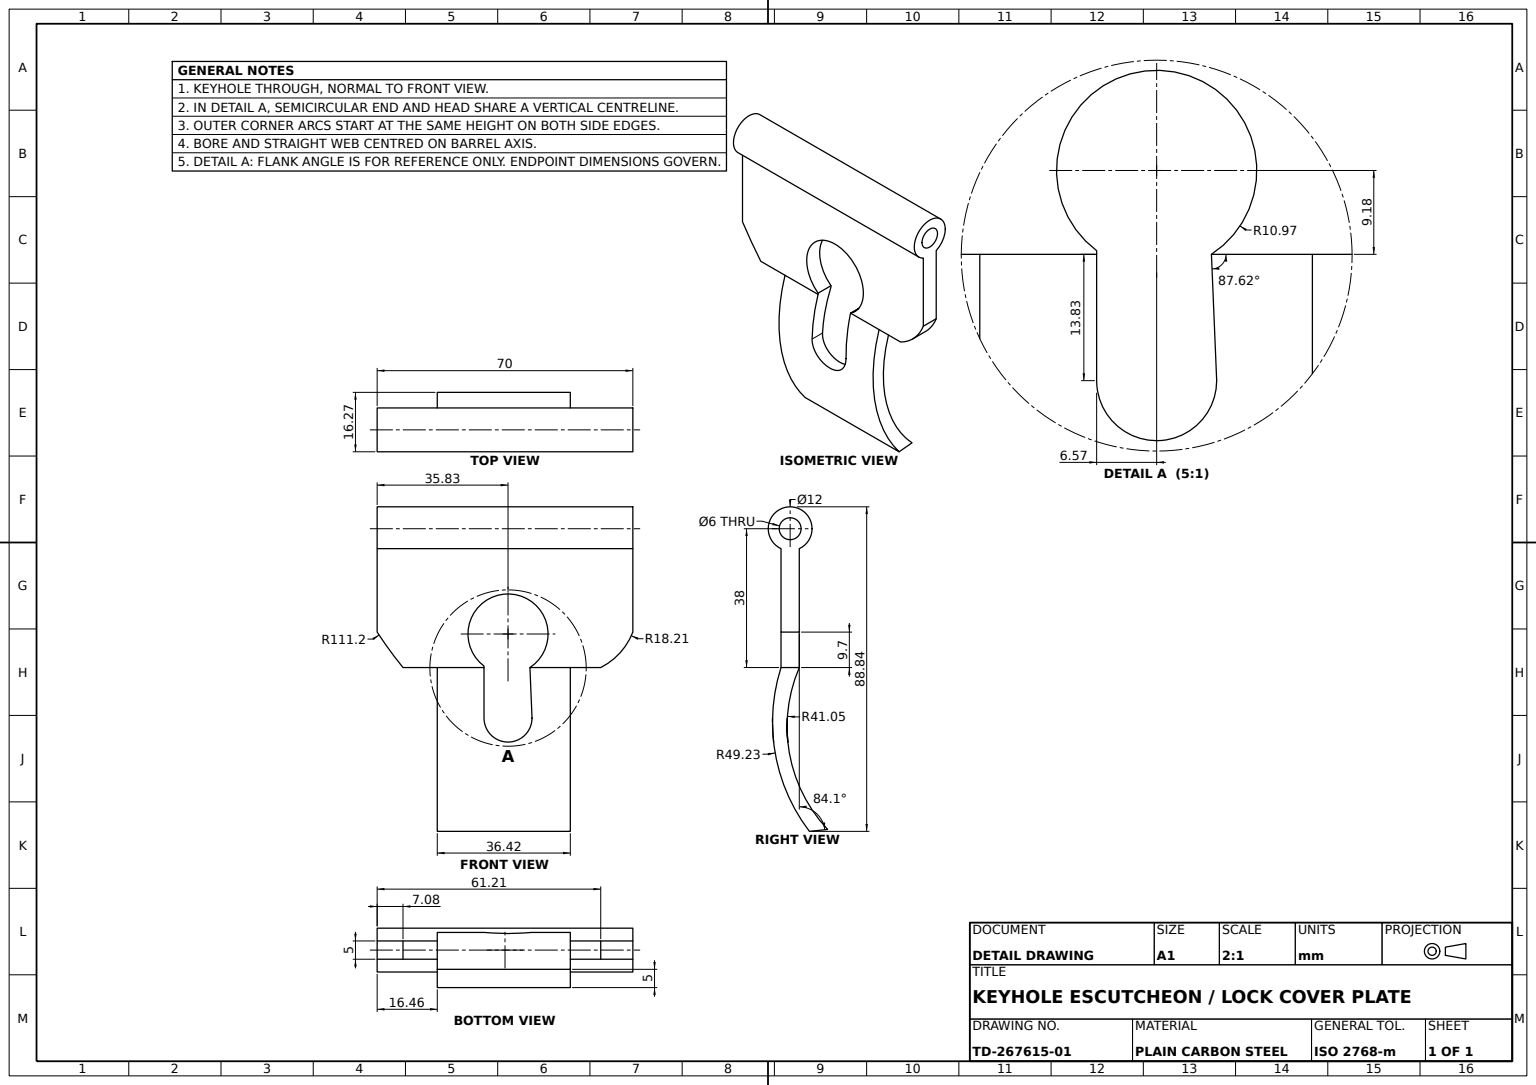
from build123d import *

# Parameters (mm, degrees)
BARREL_AND_PLATE_PROFILE_SKETCH_R = 3
BARREL_AND_PLATE_70MM_DEPTH       = 70
PLATE_PROFILE_TRIM_DEPTH          = 70
LOWER_PLATE_DEPTH                 = 63
KEYHOLE_CUT_DEPTH                 = 63
KEYHOLE_CUT_DEPTH_BACK            = 63
KEYHOLE_SKETCH_W                  = 3.828036988
KEYHOLE_SKETCH_H                  = 46.115634491
KEYHOLE_SKETCH_W_2                = 17.383946001
CORNER_CHAMFER_CUT_DEPTH          = 63
CORNER_CHAMFER_CUT_DEPTH_BACK     = 63
CORNER_CHAMFER_SKETCH_W           = 7.615823962
CORNER_CHAMFER_SKETCH_H           = 47.440125615
CURVED_LOWER_EDGE_CUT_DEPTH       = 63
CURVED_LOWER_EDGE_CUT_DEPTH_BACK  = 63


with BuildPart() as part:
    # Barrel and Plate Profile Sketch → Barrel and Plate 70mm (new body)
    with BuildSketch(Plane(origin=(0, 0, 0), x_dir=(0, 0, -1), z_dir=(1, 0, 0))):
        with BuildLine():
            Line((-2.5, -5.454356057), (-2.5, -38))
            Line((-2.5, -38), (2.5, -38))
            Line((2.5, -38), (2.5, -5.454356057))
            ThreePointArc((2.5, -5.454356057), (0, 6), (-2.5, -5.454356057))
        make_face()
        Circle(BARREL_AND_PLATE_PROFILE_SKETCH_R, mode=Mode.SUBTRACT)
    extrude(amount=BARREL_AND_PLATE_70MM_DEPTH)

    # Plate Profile Trim Sketch → Plate Profile Trim (cut)
    with BuildSketch(Plane(origin=(0, 0, -2.5), x_dir=(-1, 0, 0), z_dir=(0, 0, -1))):
        with BuildLine():
            Line((-70, -28.297812678), (-70, -38))
            Line((-70, -38), (-61.208453248, -38))
            ThreePointArc((-61.208453248, -38), (-66.50641986, -33.966420344), (-70, -28.297812678))
        make_face()
        with BuildLine():
            Line((-7.077917117, -38), (0, -38))
            Line((0, -38), (0, -28.297812678))
            ThreePointArc((0, -28.297812678), (-3.407881829, -33.244529129), (-7.077917117, -38))
        make_face()
    extrude(amount=-PLATE_PROFILE_TRIM_DEPTH, mode=Mode.SUBTRACT)

    # Lower Plate Sketch → Lower Plate (add)
    with BuildSketch(Plane(origin=(70, 0, 0), x_dir=(0, 0, -1), z_dir=(1, 0, 0))):
        with BuildLine():
            Line((5.265785985, -82.841381432), (10.265785985, -82.324852713))
            ThreePointArc((10.265785985, -82.324852713), (-0.231731323, -61.32131925), (2.5, -38))
            Line((2.5, -38), (-2.5, -38))
            ThreePointArc((-2.5, -38), (-4.109661448, -61.371910347), (5.265785985, -82.841381432))
        make_face()
    extrude(amount=-LOWER_PLATE_DEPTH)

    # Keyhole Sketch → Keyhole Cut (cut, two sides: drawn at the far end of the back side and taken through both)
    with BuildSketch(Plane.XY.offset(-KEYHOLE_CUT_DEPTH_BACK)):
        with Locations((8.914018494, -61.057817246)):
            Rectangle(KEYHOLE_SKETCH_W, KEYHOLE_SKETCH_H)
        with Locations((61.572603173, -61.057817246)):
            Rectangle(KEYHOLE_SKETCH_W_2, KEYHOLE_SKETCH_H)
    extrude(amount=KEYHOLE_CUT_DEPTH + KEYHOLE_CUT_DEPTH_BACK, mode=Mode.SUBTRACT)

    # Corner Chamfer Sketch → Corner Chamfer Cut (cut, two sides: drawn at the far end of the back side and taken through both)
    with BuildSketch(Plane.XY.offset(-CORNER_CHAMFER_CUT_DEPTH_BACK)):
        with Locations((12.649212284, -61.720062807)):
            Rectangle(CORNER_CHAMFER_SKETCH_W, CORNER_CHAMFER_SKETCH_H)
    extrude(amount=CORNER_CHAMFER_CUT_DEPTH + CORNER_CHAMFER_CUT_DEPTH_BACK, mode=Mode.SUBTRACT)

    # Curved Lower Edge Sketch → Curved Lower Edge Cut (cut, two sides: drawn at the far end of the back side and taken through both)
    with BuildSketch(Plane(origin=(0, 0, -2.5), x_dir=(-1, 0, 0), z_dir=(0, 0, -1)).offset(-CURVED_LOWER_EDGE_CUT_DEPTH_BACK)):
        with BuildLine():
            Line((-42.377724671, -51.285597096), (-42.400406488, -51.831163346))
            ThreePointArc((-42.400406488, -51.831163346), (-35.827806952, -58.403762881), (-29.255207417, -51.831163346))
            Line((-29.255207417, -51.831163346), (-29.255207417, -38))
            Line((-29.255207417, -38), (-41.825378407, -38))
            Line((-41.825378407, -38), (-42.377724671, -51.285597096))
        make_face()
        with BuildLine():
            ThreePointArc((-29.255207417, -37.597568213), (-36.178737372, -17.856631692), (-41.825378407, -38))
            Line((-41.825378407, -38), (-29.255207417, -38))
            Line((-29.255207417, -38), (-29.255207417, -37.597568213))
        make_face()
    extrude(amount=CURVED_LOWER_EDGE_CUT_DEPTH + CURVED_LOWER_EDGE_CUT_DEPTH_BACK, mode=Mode.SUBTRACT)


solid = part.part
